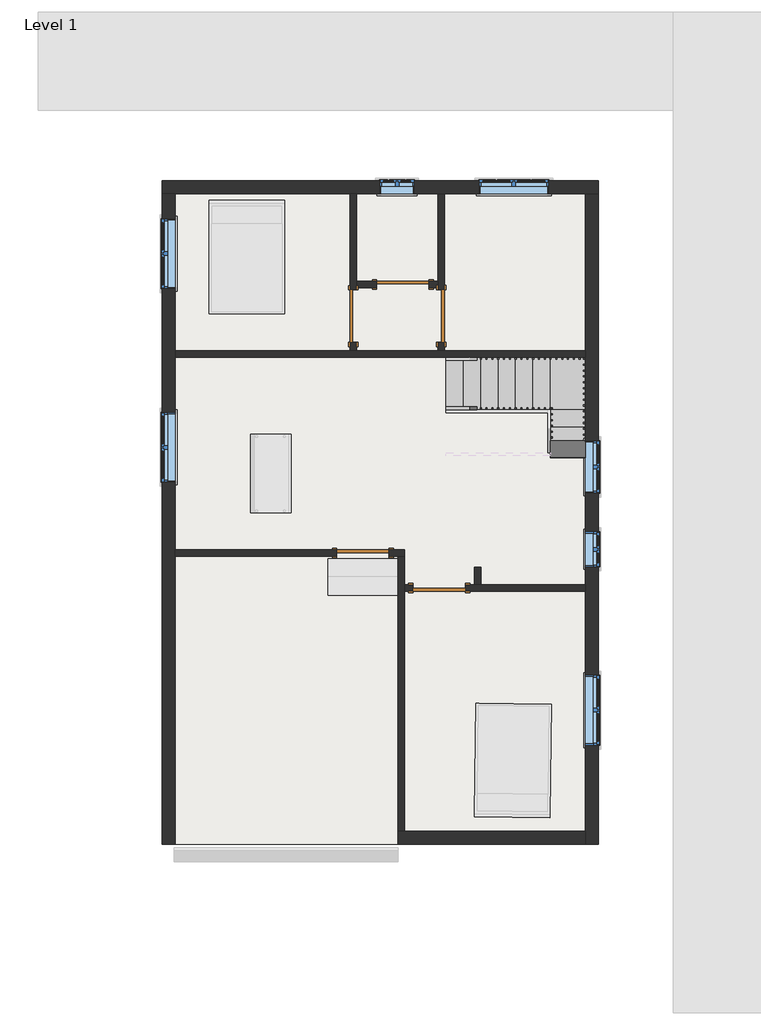
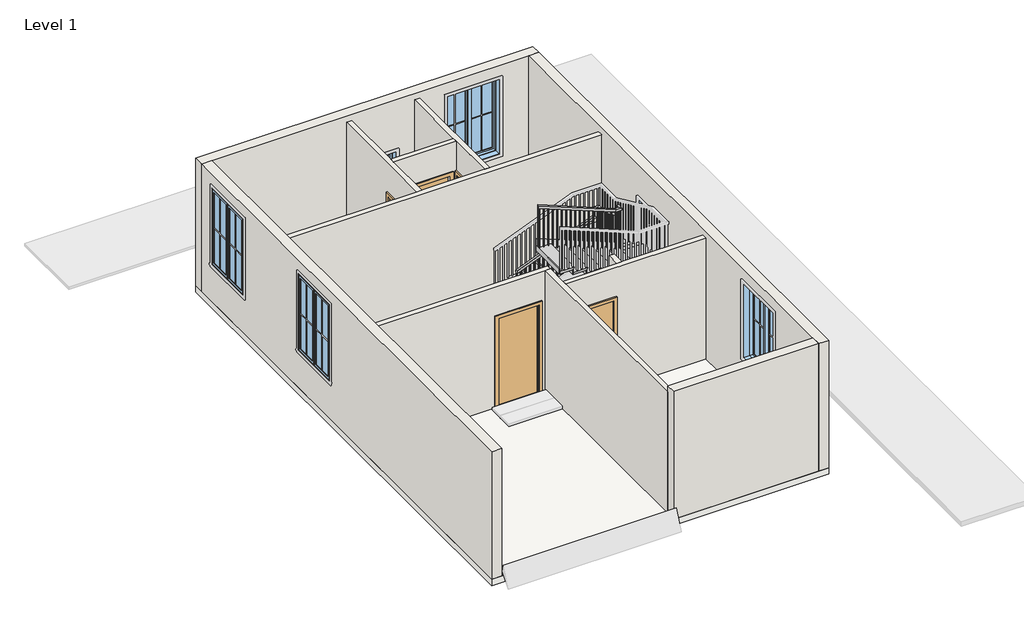
# One storey, part 1 of 2: 12 walls, 7 windows, 5 doors, 1 railing, 1 slab, 1 stair flight.
"""IFC4 building model written with IfcOpenShell, lengths in millimetres."""

from ifc_helpers import new_model, si_unit, frame, origin, origin_with_axes, place, context, project, spatial, polyline, outline, extrude, faceted_brep, transform, mapped, element, save
from components import door_e5f9f3c4, door_305aa2a5, stair_flight_8b794a03, window_c417fced, window_79f73a1a, window_6ca1769e

model = new_model("IFC4")

# Units and contexts
model_context = context("Model", 3, world=origin())
ifc_project = project(units=[si_unit("LENGTHUNIT", "METRE", prefix="MILLI")], contexts=[model_context])

# Site, building, storey
site = spatial("IfcSite", under=ifc_project)
building = spatial("IfcBuilding", under=site)
storey = spatial("IfcBuildingStorey", under=building, Name="Level 1", Elevation=0.0)

# Doors
placement = place(None, origin())
door_shape = door_e5f9f3c4(model_context)
element("IfcDoor", 1, ObjectType="Single-Flush : 36\" x 84\"", at=placement, inside=storey, context=model_context, shape_type="MappedRepresentation", body=[
    mapped(door_shape, transform((5727.7, 12245.5823212, 0.0), x_axis=(1.0, 0.0, 0.0), y_axis=(0.0, 1.0, 0.0), z_axis=(0.0, 0.0, 1.0))),
])
element("IfcDoor", 2, ObjectType="Single-Flush : 36\" x 84\"", at=placement, inside=storey, context=model_context, shape_type="MappedRepresentation", body=[
    mapped(door_shape, transform((6394.45, 11693.1323212, 0.0), x_axis=(0.0, -1.0, 0.0), y_axis=(1.0, 0.0, 0.0), z_axis=(0.0, 0.0, 1.0))),
])
element("IfcDoor", 3, ObjectType="Single-Flush : 36\" x 84\"", at=placement, inside=storey, context=model_context, shape_type="MappedRepresentation", body=[
    mapped(door_shape, transform((6362.7, 6949.6823212, 0.0), x_axis=(-1.0, 0.0, 0.0), y_axis=(0.0, -1.0, 0.0), z_axis=(0.0, 0.0, 1.0))),
])
element("IfcDoor", 4, ObjectType="Single-Flush : 36\" x 84\"", at=placement, inside=storey, context=model_context, shape_type="MappedRepresentation", body=[
    mapped(door_shape, transform((5029.2, 7559.2823212, 0.0), x_axis=(1.0, 0.0, 0.0), y_axis=(0.0, 1.0, 0.0), z_axis=(0.0, 0.0, 1.0))),
])
door_2_shape = door_305aa2a5(model_context)
element("IfcDoor", 5, ObjectType="Single-Flush : 36\" x 84\"", at=placement, inside=storey, context=model_context, shape_type="MappedRepresentation", body=[
    mapped(door_2_shape, transform((4857.75, 11689.9573212, 0.0), x_axis=(0.0, -1.0, 0.0), y_axis=(1.0, 0.0, 0.0), z_axis=(0.0, 0.0, 1.0))),
])

# Railing
element("IfcRailing", 6, ObjectType="Handrail - Rectangular", at=placement, inside=storey, context=model_context, shape_type="SolidModel", body=[
    faceted_brep([(6477.0, 10105.6323212, 1036.32), (6477.0, 10105.6323212, 981.6067256), (6477.0, 10054.8323212, 981.6067256), (6477.0, 10054.8323212, 1036.32), (8229.6, 10105.6323212, 1737.36), (8280.4, 10105.6323212, 1702.9667256), (8280.4, 10054.8323212, 1702.9667256), (8229.6, 10054.8323212, 1737.36), (8229.6, 10105.6323212, 1924.5942857), (8280.4, 10105.6323212, 1873.7942857), (8280.4, 10054.8323212, 1873.7942857), (8229.6, 10054.8323212, 1924.5942857), (8356.6, 10105.6323212, 1924.5942857), (8356.6, 10105.6323212, 1873.7942857), (8305.8, 10054.8323212, 1873.7942857), (8305.8, 10054.8323212, 1924.5942857), (8356.6, 9978.6323212, 1924.5942857), (8356.6, 9967.5713743, 1873.7942857), (8305.8, 9967.5713743, 1873.7942857), (8305.8, 9978.6323212, 1924.5942857), (8356.6, 9330.9323212, 2220.6857143), (8356.6, 9280.1323212, 2188.0521386), (8305.8, 9280.1323212, 2188.0521386), (8305.8, 9330.9323212, 2220.6857143), (8356.6, 9330.9323212, 2407.92), (8356.6, 9280.1323212, 2357.12), (8305.8, 9280.1323212, 2357.12), (8305.8, 9330.9323212, 2407.92), (8356.6, 9203.9323212, 2407.92), (8356.6, 9203.9323212, 2357.12), (8305.8, 9254.7323212, 2357.12), (8305.8, 9254.7323212, 2407.92), (8229.6, 9203.9323212, 2407.92), (8219.8168139, 9203.9323212, 2357.12), (8219.8168139, 9254.7323212, 2357.12), (8229.6, 9254.7323212, 2407.92), (6477.0, 9203.9323212, 3108.96), (6477.0, 9254.7323212, 3108.96), (6477.0, 9254.7323212, 3054.2467256), (6477.0, 9203.9323212, 3054.2467256)], [[[0, 1, 2, 3]], [[1, 0, 4, 5]], [[2, 1, 5, 6]], [[3, 2, 6, 7]], [[0, 3, 7, 4]], [[5, 4, 8, 9]], [[6, 5, 9, 10]], [[7, 6, 10, 11]], [[4, 7, 11, 8]], [[9, 8, 12, 13]], [[10, 9, 13, 14]], [[11, 10, 14, 15]], [[8, 11, 15, 12]], [[13, 12, 16, 17]], [[14, 13, 17, 18]], [[15, 14, 18, 19]], [[12, 15, 19, 16]], [[17, 16, 20, 21]], [[18, 17, 21, 22]], [[19, 18, 22, 23]], [[16, 19, 23, 20]], [[21, 20, 24, 25]], [[22, 21, 25, 26]], [[23, 22, 26, 27]], [[20, 23, 27, 24]], [[25, 24, 28, 29]], [[26, 25, 29, 30]], [[27, 26, 30, 31]], [[24, 27, 31, 28]], [[29, 28, 32, 33]], [[30, 29, 33, 34]], [[31, 30, 34, 35]], [[28, 31, 35, 32]], [[36, 37, 38, 39]], [[33, 32, 36, 39]], [[34, 33, 39, 38]], [[35, 34, 38, 37]], [[32, 35, 37, 36]]]),
    extrude(outline(polyline([(3040.2767256, 6511.925), (3047.8967256, 6492.875), (2072.64, 6492.875), (2072.64, 6511.925), (3040.2767256, 6511.925)])), frame((0.0, 9219.8073212, 0.0), z_axis=(0.0, 1.0, 0.0), x_axis=(0.0, 0.0, 1.0)), (0.0, 0.0, 1.0), 19.05),
    extrude(outline(polyline([(2999.6367256, 6613.525), (3007.2567256, 6594.475), (2072.64, 6594.475), (2072.64, 6613.525), (2999.6367256, 6613.525)])), frame((0.0, 9219.8073212, 0.0), z_axis=(0.0, 1.0, 0.0), x_axis=(0.0, 0.0, 1.0)), (0.0, 0.0, 1.0), 19.05),
    extrude(outline(polyline([(2958.9967256, 6715.125), (2966.6167256, 6696.075), (2072.64, 6696.075), (2072.64, 6715.125), (2958.9967256, 6715.125)])), frame((0.0, 9219.8073212, 0.0), z_axis=(0.0, 1.0, 0.0), x_axis=(0.0, 0.0, 1.0)), (0.0, 0.0, 1.0), 19.05),
    extrude(outline(polyline([(2918.3567256, 6816.725), (2925.9767256, 6797.675), (1950.72, 6797.675), (1950.72, 6816.725), (2918.3567256, 6816.725)])), frame((0.0, 9219.8073212, 0.0), z_axis=(0.0, 1.0, 0.0), x_axis=(0.0, 0.0, 1.0)), (0.0, 0.0, 1.0), 19.05),
    extrude(outline(polyline([(2877.7167256, 6918.325), (2885.3367256, 6899.275), (1950.72, 6899.275), (1950.72, 6918.325), (2877.7167256, 6918.325)])), frame((0.0, 9219.8073212, 0.0), z_axis=(0.0, 1.0, 0.0), x_axis=(0.0, 0.0, 1.0)), (0.0, 0.0, 1.0), 19.05),
    extrude(outline(polyline([(2837.0767256, 7019.925), (2844.6967256, 7000.875), (1950.72, 7000.875), (1950.72, 7019.925), (2837.0767256, 7019.925)])), frame((0.0, 9219.8073212, 0.0), z_axis=(0.0, 1.0, 0.0), x_axis=(0.0, 0.0, 1.0)), (0.0, 0.0, 1.0), 19.05),
    extrude(outline(polyline([(2796.4367256, 7121.525), (2804.0567256, 7102.475), (1828.8, 7102.475), (1828.8, 7121.525), (2796.4367256, 7121.525)])), frame((0.0, 9219.8073212, 0.0), z_axis=(0.0, 1.0, 0.0), x_axis=(0.0, 0.0, 1.0)), (0.0, 0.0, 1.0), 19.05),
    extrude(outline(polyline([(2755.7967256, 7223.125), (2763.4167256, 7204.075), (1828.8, 7204.075), (1828.8, 7223.125), (2755.7967256, 7223.125)])), frame((0.0, 9219.8073212, 0.0), z_axis=(0.0, 1.0, 0.0), x_axis=(0.0, 0.0, 1.0)), (0.0, 0.0, 1.0), 19.05),
    extrude(outline(polyline([(2715.1567256, 7324.725), (2722.7767256, 7305.675), (1828.8, 7305.675), (1828.8, 7324.725), (2715.1567256, 7324.725)])), frame((0.0, 9219.8073212, 0.0), z_axis=(0.0, 1.0, 0.0), x_axis=(0.0, 0.0, 1.0)), (0.0, 0.0, 1.0), 19.05),
    extrude(outline(polyline([(2674.5167256, 7426.325), (2682.1367256, 7407.275), (1706.88, 7407.275), (1706.88, 7426.325), (2674.5167256, 7426.325)])), frame((0.0, 9219.8073212, 0.0), z_axis=(0.0, 1.0, 0.0), x_axis=(0.0, 0.0, 1.0)), (0.0, 0.0, 1.0), 19.05),
    extrude(outline(polyline([(2633.8767256, 7527.925), (2641.4967256, 7508.875), (1706.88, 7508.875), (1706.88, 7527.925), (2633.8767256, 7527.925)])), frame((0.0, 9219.8073212, 0.0), z_axis=(0.0, 1.0, 0.0), x_axis=(0.0, 0.0, 1.0)), (0.0, 0.0, 1.0), 19.05),
    extrude(outline(polyline([(2593.2367256, 7629.525), (2600.8567256, 7610.475), (1706.88, 7610.475), (1706.88, 7629.525), (2593.2367256, 7629.525)])), frame((0.0, 9219.8073212, 0.0), z_axis=(0.0, 1.0, 0.0), x_axis=(0.0, 0.0, 1.0)), (0.0, 0.0, 1.0), 19.05),
    extrude(outline(polyline([(2552.5967256, 7731.125), (2560.2167256, 7712.075), (1584.96, 7712.075), (1584.96, 7731.125), (2552.5967256, 7731.125)])), frame((0.0, 9219.8073212, 0.0), z_axis=(0.0, 1.0, 0.0), x_axis=(0.0, 0.0, 1.0)), (0.0, 0.0, 1.0), 19.05),
    extrude(outline(polyline([(2511.9567256, 7832.725), (2519.5767256, 7813.675), (1584.96, 7813.675), (1584.96, 7832.725), (2511.9567256, 7832.725)])), frame((0.0, 9219.8073212, 0.0), z_axis=(0.0, 1.0, 0.0), x_axis=(0.0, 0.0, 1.0)), (0.0, 0.0, 1.0), 19.05),
    extrude(outline(polyline([(2471.3167256, 7934.325), (2478.9367256, 7915.275), (1584.96, 7915.275), (1584.96, 7934.325), (2471.3167256, 7934.325)])), frame((0.0, 9219.8073212, 0.0), z_axis=(0.0, 1.0, 0.0), x_axis=(0.0, 0.0, 1.0)), (0.0, 0.0, 1.0), 19.05),
    extrude(outline(polyline([(2430.6767256, 8035.925), (2438.2967256, 8016.875), (1463.04, 8016.875), (1463.04, 8035.925), (2430.6767256, 8035.925)])), frame((0.0, 9219.8073212, 0.0), z_axis=(0.0, 1.0, 0.0), x_axis=(0.0, 0.0, 1.0)), (0.0, 0.0, 1.0), 19.05),
    extrude(outline(polyline([(2390.0367256, 8137.525), (2397.6567256, 8118.475), (1463.04, 8118.475), (1463.04, 8137.525), (2390.0367256, 8137.525)])), frame((0.0, 9219.8073212, 0.0), z_axis=(0.0, 1.0, 0.0), x_axis=(0.0, 0.0, 1.0)), (0.0, 0.0, 1.0), 19.05),
    extrude(outline(polyline([(2349.3967256, 8239.125), (2357.0167256, 8220.075), (1463.04, 8220.075), (1463.04, 8239.125), (2349.3967256, 8239.125)])), frame((0.0, 9219.8073212, 0.0), z_axis=(0.0, 1.0, 0.0), x_axis=(0.0, 0.0, 1.0)), (0.0, 0.0, 1.0), 19.05),
    extrude(outline(polyline([(8321.675, 9276.9573212), (8340.725, 9276.9573212), (8340.725, 9257.9073212), (8321.675, 9257.9073212), (8321.675, 9276.9573212)])), frame((0.0, 0.0, 1219.2), z_axis=(0.0, 0.0, 1.0), x_axis=(1.0, 0.0, 0.0)), (0.0, 0.0, 1.0), 1137.92),
    extrude(outline(polyline([(9359.5073212, 2151.7664243), (9378.5573212, 2143.0578528), (9378.5573212, 1219.2), (9359.5073212, 1219.2), (9359.5073212, 2151.7664243)])), frame((8321.675, 0.0, 0.0), z_axis=(1.0, 0.0, 0.0), x_axis=(0.0, 1.0, 0.0)), (0.0, 0.0, 1.0), 19.05),
    extrude(outline(polyline([(9461.1073212, 2105.32071), (9480.1573212, 2096.6121386), (9480.1573212, 1219.2), (9461.1073212, 1219.2), (9461.1073212, 2105.32071)])), frame((8321.675, 0.0, 0.0), z_axis=(1.0, 0.0, 0.0), x_axis=(0.0, 1.0, 0.0)), (0.0, 0.0, 1.0), 19.05),
    extrude(outline(polyline([(9562.7073212, 2058.8749957), (9581.7573212, 2050.1664243), (9581.7573212, 1097.28), (9562.7073212, 1097.28), (9562.7073212, 2058.8749957)])), frame((8321.675, 0.0, 0.0), z_axis=(1.0, 0.0, 0.0), x_axis=(0.0, 1.0, 0.0)), (0.0, 0.0, 1.0), 19.05),
    extrude(outline(polyline([(9664.3073212, 2012.4292814), (9683.3573212, 2003.72071), (9683.3573212, 1097.28), (9664.3073212, 1097.28), (9664.3073212, 2012.4292814)])), frame((8321.675, 0.0, 0.0), z_axis=(1.0, 0.0, 0.0), x_axis=(0.0, 1.0, 0.0)), (0.0, 0.0, 1.0), 19.05),
    extrude(outline(polyline([(9765.9073212, 1965.9835671), (9784.9573212, 1957.2749957), (9784.9573212, 975.36), (9765.9073212, 975.36), (9765.9073212, 1965.9835671)])), frame((8321.675, 0.0, 0.0), z_axis=(1.0, 0.0, 0.0), x_axis=(0.0, 1.0, 0.0)), (0.0, 0.0, 1.0), 19.05),
    extrude(outline(polyline([(9867.5073212, 1919.5378528), (9886.5573212, 1910.8292814), (9886.5573212, 975.36), (9867.5073212, 975.36), (9867.5073212, 1919.5378528)])), frame((8321.675, 0.0, 0.0), z_axis=(1.0, 0.0, 0.0), x_axis=(0.0, 1.0, 0.0)), (0.0, 0.0, 1.0), 19.05),
    extrude(outline(polyline([(9969.1073212, 1873.0921386), (9988.1573212, 1864.3835671), (9988.1573212, 975.36), (9969.1073212, 975.36), (9969.1073212, 1873.0921386)])), frame((8321.675, 0.0, 0.0), z_axis=(1.0, 0.0, 0.0), x_axis=(0.0, 1.0, 0.0)), (0.0, 0.0, 1.0), 19.05),
    extrude(outline(polyline([(8296.275, 10070.7073212), (8296.275, 10089.7573212), (8315.325, 10089.7573212), (8315.325, 10070.7073212), (8296.275, 10070.7073212)])), frame((0.0, 0.0, 853.44), z_axis=(0.0, 0.0, 1.0), x_axis=(1.0, 0.0, 0.0)), (0.0, 0.0, 1.0), 1020.3542857),
    extrude(outline(polyline([(1676.2967256, 8213.725), (1668.6767256, 8194.675), (731.52, 8194.675), (731.52, 8213.725), (1676.2967256, 8213.725)])), frame((0.0, 10070.7073212, 0.0), z_axis=(0.0, 1.0, 0.0), x_axis=(0.0, 0.0, 1.0)), (0.0, 0.0, 1.0), 19.05),
    extrude(outline(polyline([(1635.6567256, 8112.125), (1628.0367256, 8093.075), (731.52, 8093.075), (731.52, 8112.125), (1635.6567256, 8112.125)])), frame((0.0, 10070.7073212, 0.0), z_axis=(0.0, 1.0, 0.0), x_axis=(0.0, 0.0, 1.0)), (0.0, 0.0, 1.0), 19.05),
    extrude(outline(polyline([(1595.0167256, 8010.525), (1587.3967256, 7991.475), (731.52, 7991.475), (731.52, 8010.525), (1595.0167256, 8010.525)])), frame((0.0, 10070.7073212, 0.0), z_axis=(0.0, 1.0, 0.0), x_axis=(0.0, 0.0, 1.0)), (0.0, 0.0, 1.0), 19.05),
    extrude(outline(polyline([(1554.3767256, 7908.925), (1546.7567256, 7889.875), (609.6, 7889.875), (609.6, 7908.925), (1554.3767256, 7908.925)])), frame((0.0, 10070.7073212, 0.0), z_axis=(0.0, 1.0, 0.0), x_axis=(0.0, 0.0, 1.0)), (0.0, 0.0, 1.0), 19.05),
    extrude(outline(polyline([(1513.7367256, 7807.325), (1506.1167256, 7788.275), (609.6, 7788.275), (609.6, 7807.325), (1513.7367256, 7807.325)])), frame((0.0, 10070.7073212, 0.0), z_axis=(0.0, 1.0, 0.0), x_axis=(0.0, 0.0, 1.0)), (0.0, 0.0, 1.0), 19.05),
    extrude(outline(polyline([(1473.0967256, 7705.725), (1465.4767256, 7686.675), (609.6, 7686.675), (609.6, 7705.725), (1473.0967256, 7705.725)])), frame((0.0, 10070.7073212, 0.0), z_axis=(0.0, 1.0, 0.0), x_axis=(0.0, 0.0, 1.0)), (0.0, 0.0, 1.0), 19.05),
    extrude(outline(polyline([(1432.4567256, 7604.125), (1424.8367256, 7585.075), (487.68, 7585.075), (487.68, 7604.125), (1432.4567256, 7604.125)])), frame((0.0, 10070.7073212, 0.0), z_axis=(0.0, 1.0, 0.0), x_axis=(0.0, 0.0, 1.0)), (0.0, 0.0, 1.0), 19.05),
    extrude(outline(polyline([(1391.8167256, 7502.525), (1384.1967256, 7483.475), (487.68, 7483.475), (487.68, 7502.525), (1391.8167256, 7502.525)])), frame((0.0, 10070.7073212, 0.0), z_axis=(0.0, 1.0, 0.0), x_axis=(0.0, 0.0, 1.0)), (0.0, 0.0, 1.0), 19.05),
    extrude(outline(polyline([(1351.1767256, 7400.925), (1343.5567256, 7381.875), (487.68, 7381.875), (487.68, 7400.925), (1351.1767256, 7400.925)])), frame((0.0, 10070.7073212, 0.0), z_axis=(0.0, 1.0, 0.0), x_axis=(0.0, 0.0, 1.0)), (0.0, 0.0, 1.0), 19.05),
    extrude(outline(polyline([(1310.5367256, 7299.325), (1302.9167256, 7280.275), (365.76, 7280.275), (365.76, 7299.325), (1310.5367256, 7299.325)])), frame((0.0, 10070.7073212, 0.0), z_axis=(0.0, 1.0, 0.0), x_axis=(0.0, 0.0, 1.0)), (0.0, 0.0, 1.0), 19.05),
    extrude(outline(polyline([(1269.8967256, 7197.725), (1262.2767256, 7178.675), (365.76, 7178.675), (365.76, 7197.725), (1269.8967256, 7197.725)])), frame((0.0, 10070.7073212, 0.0), z_axis=(0.0, 1.0, 0.0), x_axis=(0.0, 0.0, 1.0)), (0.0, 0.0, 1.0), 19.05),
    extrude(outline(polyline([(1229.2567256, 7096.125), (1221.6367256, 7077.075), (365.76, 7077.075), (365.76, 7096.125), (1229.2567256, 7096.125)])), frame((0.0, 10070.7073212, 0.0), z_axis=(0.0, 1.0, 0.0), x_axis=(0.0, 0.0, 1.0)), (0.0, 0.0, 1.0), 19.05),
    extrude(outline(polyline([(1188.6167256, 6994.525), (1180.9967256, 6975.475), (243.84, 6975.475), (243.84, 6994.525), (1188.6167256, 6994.525)])), frame((0.0, 10070.7073212, 0.0), z_axis=(0.0, 1.0, 0.0), x_axis=(0.0, 0.0, 1.0)), (0.0, 0.0, 1.0), 19.05),
    extrude(outline(polyline([(1147.9767256, 6892.925), (1140.3567256, 6873.875), (243.84, 6873.875), (243.84, 6892.925), (1147.9767256, 6892.925)])), frame((0.0, 10070.7073212, 0.0), z_axis=(0.0, 1.0, 0.0), x_axis=(0.0, 0.0, 1.0)), (0.0, 0.0, 1.0), 19.05),
    extrude(outline(polyline([(1107.3367256, 6791.325), (1099.7167256, 6772.275), (243.84, 6772.275), (243.84, 6791.325), (1107.3367256, 6791.325)])), frame((0.0, 10070.7073212, 0.0), z_axis=(0.0, 1.0, 0.0), x_axis=(0.0, 0.0, 1.0)), (0.0, 0.0, 1.0), 19.05),
    extrude(outline(polyline([(1066.6967256, 6689.725), (1059.0767256, 6670.675), (121.92, 6670.675), (121.92, 6689.725), (1066.6967256, 6689.725)])), frame((0.0, 10070.7073212, 0.0), z_axis=(0.0, 1.0, 0.0), x_axis=(0.0, 0.0, 1.0)), (0.0, 0.0, 1.0), 19.05),
    extrude(outline(polyline([(1026.0567256, 6588.125), (1018.4367256, 6569.075), (121.92, 6569.075), (121.92, 6588.125), (1026.0567256, 6588.125)])), frame((0.0, 10070.7073212, 0.0), z_axis=(0.0, 1.0, 0.0), x_axis=(0.0, 0.0, 1.0)), (0.0, 0.0, 1.0), 19.05),
    extrude(outline(polyline([(8321.675, 9238.8573212), (8340.725, 9238.8573212), (8340.725, 9219.8073212), (8321.675, 9219.8073212), (8321.675, 9238.8573212)])), frame((0.0, 0.0, 1341.12), z_axis=(0.0, 0.0, 1.0), x_axis=(1.0, 0.0, 0.0)), (0.0, 0.0, 1.0), 1016.0),
    extrude(outline(polyline([(8321.675, 10070.7073212), (8321.675, 10089.7573212), (8340.725, 10089.7573212), (8340.725, 10070.7073212), (8321.675, 10070.7073212)])), frame((0.0, 0.0, 853.44), z_axis=(0.0, 0.0, 1.0), x_axis=(1.0, 0.0, 0.0)), (0.0, 0.0, 1.0), 1020.3542857),
    extrude(outline(polyline([(3046.6267256, 6496.05), (3054.2467256, 6477.0), (2072.64, 6477.0), (2072.64, 6496.05), (3046.6267256, 6496.05)])), frame((0.0, 9219.8073212, 0.0), z_axis=(0.0, 1.0, 0.0), x_axis=(0.0, 0.0, 1.0)), (0.0, 0.0, 1.0), 19.05),
    extrude(outline(polyline([(989.2267256, 6496.05), (981.6067256, 6477.0), (121.92, 6477.0), (121.92, 6496.05), (989.2267256, 6496.05)])), frame((0.0, 10070.7073212, 0.0), z_axis=(0.0, 1.0, 0.0), x_axis=(0.0, 0.0, 1.0)), (0.0, 0.0, 1.0), 19.05),
])

# Slab
element("IfcSlab", 7, ObjectType="Generic - 12\"", at=placement, inside=storey, context=model_context, shape_type="SweptSolid", body=[
    extrude(outline(polyline([(9144.0, 14055.3323212), (9144.0, 2472.9323212), (1524.0, 2472.9323212), (1524.0, 14055.3323212), (9144.0, 14055.3323212)])), frame((0.0, 0.0, -152.4), z_axis=(0.0, 0.0, 1.0), x_axis=(1.0, 0.0, 0.0)), (0.0, 0.0, 1.0), 152.4),
])

# Stair flight
stair_flight_shape = stair_flight_8b794a03(model_context)
element("IfcStairFlight", 8, ObjectType="2\" Tread 1\" Nosing 1/4\" Riser", at=placement, inside=storey, context=model_context, shape_type="MappedRepresentation", body=[
    mapped(stair_flight_shape, transform((0.0, 0.0, 0.0), x_axis=(1.0, 0.0, 0.0), y_axis=(0.0, 1.0, 0.0), z_axis=(0.0, 0.0, 1.0))),
])

# Walls
element("IfcWall", 9, ObjectType="Generic - 5\"", at=placement, inside=storey, context=model_context, shape_type="Brep", body=[
    faceted_brep([(4800.6, 11232.7573212, 2133.6), (4800.6, 11232.7573212, 0.0), (4800.6, 11083.5323212, 0.0), (4800.6, 11083.5323212, 2895.6), (4800.6, 13826.7323212, 2895.6), (4800.6, 13826.7323212, 0.0), (4800.6, 12147.1573212, 0.0), (4800.6, 12147.1573212, 2133.6), (4914.9, 11083.5323212, 0.0), (4914.9, 11232.7573212, 0.0), (4914.9, 11232.7573212, 2133.6), (4914.9, 12147.1573212, 2133.6), (4914.9, 12147.1573212, 0.0), (4914.9, 12188.4323212, 0.0), (4914.9, 12302.7323212, 0.0), (4914.9, 13826.7323212, 0.0), (4914.9, 13826.7323212, 2895.6), (4914.9, 12302.7323212, 2895.6), (4914.9, 12188.4323212, 2895.6), (4914.9, 11083.5323212, 2895.6)], [[[0, 1, 2, 3, 4, 5, 6, 7]], [[8, 9, 10, 11, 12, 13, 14, 15, 16, 17, 18, 19]], [[6, 5, 15, 14, 13, 12]], [[2, 1, 9, 8]], [[5, 4, 16, 15]], [[3, 2, 8, 19]], [[10, 9, 1, 0]], [[11, 10, 0, 7]], [[12, 11, 7, 6]], [[4, 3, 19, 18, 17, 16]]]),
])
element("IfcWall", 10, ObjectType="Generic - 5\"", at=placement, inside=storey, context=model_context, shape_type="Brep", body=[
    faceted_brep([(6337.3, 11235.9323212, 2133.6), (6337.3, 11235.9323212, 0.0), (6337.3, 11083.5323212, 0.0), (6337.3, 11083.5323212, 2895.6), (6337.3, 12188.4323212, 2895.6), (6337.3, 12302.7323212, 2895.6), (6337.3, 13826.7323212, 2895.6), (6337.3, 13826.7323212, 0.0), (6337.3, 12302.7323212, 0.0), (6337.3, 12188.4323212, 0.0), (6337.3, 12150.3323212, 0.0), (6337.3, 12150.3323212, 2133.6), (6451.6, 11083.5323212, 0.0), (6451.6, 11235.9323212, 0.0), (6451.6, 11235.9323212, 2133.6), (6451.6, 12150.3323212, 2133.6), (6451.6, 12150.3323212, 0.0), (6451.6, 13826.7323212, 0.0), (6451.6, 13826.7323212, 2895.6), (6451.6, 11083.5323212, 2895.6)], [[[0, 1, 2, 3, 4, 5, 6, 7, 8, 9, 10, 11]], [[12, 13, 14, 15, 16, 17, 18, 19]], [[2, 1, 13, 12]], [[10, 9, 8, 7, 17, 16]], [[7, 6, 18, 17]], [[3, 2, 12, 19]], [[14, 13, 1, 0]], [[15, 14, 0, 11]], [[16, 15, 11, 10]], [[6, 5, 4, 3, 19, 18]]]),
])
element("IfcWall", 11, ObjectType="Generic - 5\"", at=placement, inside=storey, context=model_context, shape_type="SweptSolid", body=[
    extrude(outline(polyline([(2133.6, 6184.9), (0.0, 6184.9), (0.0, 6337.3), (2895.6, 6337.3), (2895.6, 4914.9), (0.0, 4914.9), (0.0, 5270.5), (2133.6, 5270.5), (2133.6, 6184.9)])), frame((0.0, 12188.4323212, 0.0), z_axis=(0.0, 1.0, 0.0), x_axis=(0.0, 0.0, 1.0)), (0.0, 0.0, 1.0), 114.3),
])
element("IfcWall", 12, ObjectType="Generic - 5\"", at=placement, inside=storey, context=model_context, shape_type="Brep", body=[
    faceted_brep([(1752.6, 10969.2323212, 0.0), (8915.4, 10969.2323212, 0.0), (8915.4, 10969.2323212, 2895.6), (1752.6, 10969.2323212, 2895.6), (1752.6, 11083.5323212, 0.0), (1752.6, 11083.5323212, 2895.6), (4800.6, 11083.5323212, 2895.6), (4914.9, 11083.5323212, 2895.6), (6337.3, 11083.5323212, 2895.6), (6451.6, 11083.5323212, 2895.6), (8915.4, 11083.5323212, 2895.6), (8915.4, 11083.5323212, 0.0), (6451.6, 11083.5323212, 0.0), (6337.3, 11083.5323212, 0.0), (4914.9, 11083.5323212, 0.0), (4800.6, 11083.5323212, 0.0)], [[[0, 1, 2, 3]], [[4, 5, 6, 7, 8, 9, 10, 11, 12, 13, 14, 15]], [[1, 0, 4, 15, 14, 13, 12, 11]], [[2, 1, 11, 10]], [[0, 3, 5, 4]], [[3, 2, 10, 9, 8, 7, 6, 5]]]),
])
element("IfcWall", 13, ObjectType="Generic - 5\"", at=placement, inside=storey, context=model_context, shape_type="Brep", body=[
    faceted_brep([(5486.4, 7502.1323212, 2133.6), (5486.4, 7502.1323212, 0.0), (5638.8, 7502.1323212, 0.0), (5753.1, 7502.1323212, 0.0), (5753.1, 7502.1323212, 2895.6), (5638.8, 7502.1323212, 2895.6), (1752.6, 7502.1323212, 2895.6), (1752.6, 7502.1323212, 0.0), (4572.0, 7502.1323212, 0.0), (4572.0, 7502.1323212, 2133.6), (5753.1, 7616.4323212, 0.0), (5486.4, 7616.4323212, 0.0), (5486.4, 7616.4323212, 2133.6), (4572.0, 7616.4323212, 2133.6), (4572.0, 7616.4323212, 0.0), (1752.6, 7616.4323212, 0.0), (1752.6, 7616.4323212, 2895.6), (5753.1, 7616.4323212, 2895.6)], [[[0, 1, 2, 3, 4, 5, 6, 7, 8, 9]], [[10, 11, 12, 13, 14, 15, 16, 17]], [[8, 7, 15, 14]], [[3, 2, 1, 11, 10]], [[7, 6, 16, 15]], [[4, 3, 10, 17]], [[12, 11, 1, 0]], [[13, 12, 0, 9]], [[14, 13, 9, 8]], [[6, 5, 4, 17, 16]]]),
])
element("IfcWall", 14, ObjectType="Generic - 5\"", at=placement, inside=storey, context=model_context, shape_type="Brep", body=[
    faceted_brep([(5638.8, 7502.1323212, 0.0), (5638.8, 2700.7084466, 0.0), (5638.8, 2700.7084466, 2895.6), (5638.8, 7502.1323212, 2895.6), (5753.1, 7502.1323212, 0.0), (5753.1, 7502.1323212, 2895.6), (5753.1, 7006.8323212, 2895.6), (5753.1, 6892.5323212, 2895.6), (5753.1, 2700.7084466, 2895.6), (5753.1, 2700.7084466, 0.0), (5753.1, 6892.5323212, 0.0), (5753.1, 7006.8323212, 0.0)], [[[0, 1, 2, 3]], [[4, 5, 6, 7, 8, 9, 10, 11]], [[1, 0, 4, 11, 10, 9]], [[0, 3, 5, 4]], [[2, 1, 9, 8]], [[3, 2, 8, 7, 6, 5]]]),
])
element("IfcWall", 15, ObjectType="Generic - 5\"", at=placement, inside=storey, context=model_context, shape_type="Brep", body=[
    faceted_brep([(5905.5, 7006.8323212, 2133.6), (5905.5, 7006.8323212, 0.0), (5753.1, 7006.8323212, 0.0), (5753.1, 7006.8323212, 2895.6), (6972.3, 7006.8323212, 2895.6), (7086.6, 7006.8323212, 2895.6), (8915.4, 7006.8323212, 2895.6), (8915.4, 7006.8323212, 0.0), (7086.6, 7006.8323212, 0.0), (6972.3, 7006.8323212, 0.0), (6819.9, 7006.8323212, 0.0), (6819.9, 7006.8323212, 2133.6), (5753.1, 6892.5323212, 0.0), (5905.5, 6892.5323212, 0.0), (5905.5, 6892.5323212, 2133.6), (6819.9, 6892.5323212, 2133.6), (6819.9, 6892.5323212, 0.0), (8915.4, 6892.5323212, 0.0), (8915.4, 6892.5323212, 2895.6), (5753.1, 6892.5323212, 2895.6)], [[[0, 1, 2, 3, 4, 5, 6, 7, 8, 9, 10, 11]], [[12, 13, 14, 15, 16, 17, 18, 19]], [[2, 1, 13, 12]], [[10, 9, 8, 7, 17, 16]], [[7, 6, 18, 17]], [[3, 2, 12, 19]], [[14, 13, 1, 0]], [[15, 14, 0, 11]], [[16, 15, 11, 10]], [[6, 5, 4, 3, 19, 18]]]),
])
element("IfcWall", 16, ObjectType="Generic - 5\"", at=placement, inside=storey, context=model_context, shape_type="SweptSolid", body=[
    extrude(outline(polyline([(7086.6, 7311.6323212), (7086.6, 7006.8323212), (6972.3, 7006.8323212), (6972.3, 7311.6323212), (7086.6, 7311.6323212)])), origin_with_axes(), (0.0, 0.0, 1.0), 2895.6),
])
element("IfcWall", 17, ObjectType="Generic - 8\"", at=placement, inside=storey, context=model_context, shape_type="Brep", body=[
    faceted_brep([(1524.0, 13826.7323212, 0.0), (1752.6, 13826.7323212, 0.0), (4800.6, 13826.7323212, 0.0), (4914.9, 13826.7323212, 0.0), (6337.3, 13826.7323212, 0.0), (6451.6, 13826.7323212, 0.0), (8915.4, 13826.7323212, 0.0), (9144.0, 13826.7323212, 0.0), (9144.0, 13826.7323212, 3048.0), (8915.4, 13826.7323212, 3048.0), (1752.6, 13826.7323212, 3048.0), (1524.0, 13826.7323212, 3048.0), (8274.05, 13826.7323212, 2743.2), (8274.05, 13826.7323212, 914.4), (7054.85, 13826.7323212, 914.4), (7054.85, 13826.7323212, 2743.2), (5930.9, 13826.7323212, 1828.8), (5930.9, 13826.7323212, 914.4), (5321.3, 13826.7323212, 914.4), (5321.3, 13826.7323212, 1828.8), (1524.0, 14055.3323212, 0.0), (1524.0, 14055.3323212, 3048.0), (9144.0, 14055.3323212, 3048.0), (9144.0, 14055.3323212, 0.0), (8274.05, 14055.3323212, 2743.2), (7054.85, 14055.3323212, 2743.2), (7054.85, 14055.3323212, 914.4), (8274.05, 14055.3323212, 914.4), (5930.9, 14055.3323212, 1828.8), (5321.3, 14055.3323212, 1828.8), (5321.3, 14055.3323212, 914.4), (5930.9, 14055.3323212, 914.4)], [[[0, 1, 2, 3, 4, 5, 6, 7, 8, 9, 10, 11], [12, 13, 14, 15], [16, 17, 18, 19]], [[20, 21, 22, 23], [24, 25, 26, 27], [28, 29, 30, 31]], [[7, 6, 5, 4, 3, 2, 1, 0, 20, 23]], [[11, 10, 9, 8, 22, 21]], [[8, 7, 23, 22]], [[0, 11, 21, 20]], [[13, 12, 24, 27]], [[14, 13, 27, 26]], [[15, 14, 26, 25]], [[12, 15, 25, 24]], [[17, 16, 28, 31]], [[18, 17, 31, 30]], [[19, 18, 30, 29]], [[16, 19, 29, 28]]]),
])
element("IfcWall", 18, ObjectType="Generic - 8\"", at=placement, inside=storey, context=model_context, shape_type="Brep", body=[
    faceted_brep([(8915.4, 13826.7323212, 0.0), (8915.4, 11083.5323212, 0.0), (8915.4, 10969.2323212, 0.0), (8915.4, 7006.8323212, 0.0), (8915.4, 6892.5323212, 0.0), (8915.4, 2700.7084466, 0.0), (8915.4, 2472.1084466, 0.0), (8915.4, 2472.1084466, 3048.0), (8915.4, 2700.7084466, 3048.0), (8915.4, 13826.7323212, 3048.0), (8915.4, 4206.4823212, 2743.2), (8915.4, 4206.4823212, 914.4), (8915.4, 5425.6823212, 914.4), (8915.4, 5425.6823212, 2743.2), (8915.4, 7315.6010712, 1828.8), (8915.4, 7315.6010712, 914.4), (8915.4, 7925.2010712, 914.4), (8915.4, 7925.2010712, 1828.8), (8915.4, 8602.8899384, 2260.6), (8915.4, 8602.8899384, 914.4), (8915.4, 9517.2899384, 914.4), (8915.4, 9517.2899384, 2260.6), (9144.0, 13826.7323212, 0.0), (9144.0, 13826.7323212, 3048.0), (9144.0, 2472.1084466, 3048.0), (9144.0, 2472.1084466, 0.0), (9144.0, 4206.4823212, 2743.2), (9144.0, 5425.6823212, 2743.2), (9144.0, 5425.6823212, 914.4), (9144.0, 4206.4823212, 914.4), (9144.0, 7315.6010712, 1828.8), (9144.0, 7925.2010712, 1828.8), (9144.0, 7925.2010712, 914.4), (9144.0, 7315.6010712, 914.4), (9144.0, 8602.8899384, 2260.6), (9144.0, 9517.2899384, 2260.6), (9144.0, 9517.2899384, 914.4), (9144.0, 8602.8899384, 914.4)], [[[0, 1, 2, 3, 4, 5, 6, 7, 8, 9], [10, 11, 12, 13], [14, 15, 16, 17], [18, 19, 20, 21]], [[22, 23, 24, 25], [26, 27, 28, 29], [30, 31, 32, 33], [34, 35, 36, 37]], [[6, 5, 4, 3, 2, 1, 0, 22, 25]], [[9, 8, 7, 24, 23]], [[0, 9, 23, 22]], [[7, 6, 25, 24]], [[11, 10, 26, 29]], [[12, 11, 29, 28]], [[13, 12, 28, 27]], [[10, 13, 27, 26]], [[15, 14, 30, 33]], [[16, 15, 33, 32]], [[17, 16, 32, 31]], [[14, 17, 31, 30]], [[19, 18, 34, 37]], [[20, 19, 37, 36]], [[21, 20, 36, 35]], [[18, 21, 35, 34]]]),
])
element("IfcWall", 19, ObjectType="Generic - 8\"", at=placement, inside=storey, context=model_context, shape_type="Brep", body=[
    faceted_brep([(8915.4, 2700.7084466, 0.0), (5753.1, 2700.7084466, 0.0), (5638.8, 2700.7084466, 0.0), (5638.8, 2700.7084466, 2895.6), (5638.8, 2700.7084466, 3048.0), (8915.4, 2700.7084466, 3048.0), (8915.4, 2472.1084466, 0.0), (8915.4, 2472.1084466, 3048.0), (5638.8, 2472.1084466, 3048.0), (5638.8, 2472.1084466, 0.0)], [[[0, 1, 2, 3, 4, 5]], [[6, 7, 8, 9]], [[2, 1, 0, 6, 9]], [[4, 3, 2, 9, 8]], [[5, 4, 8, 7]], [[0, 5, 7, 6]]]),
])
element("IfcWall", 20, ObjectType="Generic - 8\"", at=placement, inside=storey, context=model_context, shape_type="Brep", body=[
    faceted_brep([(1752.6, 2472.9323212, 0.0), (1752.6, 7502.1323212, 0.0), (1752.6, 7616.4323212, 0.0), (1752.6, 10969.2323212, 0.0), (1752.6, 11083.5323212, 0.0), (1752.6, 13826.7323212, 0.0), (1752.6, 13826.7323212, 3048.0), (1752.6, 2472.9323212, 3048.0), (1752.6, 13390.2194306, 2743.2), (1752.6, 13390.2194306, 914.4), (1752.6, 12171.0194306, 914.4), (1752.6, 12171.0194306, 2743.2), (1752.6, 10010.3823212, 2743.2), (1752.6, 10010.3823212, 914.4), (1752.6, 8791.1823212, 914.4), (1752.6, 8791.1823212, 2743.2), (1524.0, 2472.9323212, 0.0), (1524.0, 2472.9323212, 3048.0), (1524.0, 13826.7323212, 3048.0), (1524.0, 13826.7323212, 0.0), (1524.0, 13390.2194306, 2743.2), (1524.0, 12171.0194306, 2743.2), (1524.0, 12171.0194306, 914.4), (1524.0, 13390.2194306, 914.4), (1524.0, 10010.3823212, 2743.2), (1524.0, 8791.1823212, 2743.2), (1524.0, 8791.1823212, 914.4), (1524.0, 10010.3823212, 914.4)], [[[0, 1, 2, 3, 4, 5, 6, 7], [8, 9, 10, 11], [12, 13, 14, 15]], [[16, 17, 18, 19], [20, 21, 22, 23], [24, 25, 26, 27]], [[5, 4, 3, 2, 1, 0, 16, 19]], [[7, 6, 18, 17]], [[0, 7, 17, 16]], [[6, 5, 19, 18]], [[9, 8, 20, 23]], [[10, 9, 23, 22]], [[11, 10, 22, 21]], [[8, 11, 21, 20]], [[13, 12, 24, 27]], [[14, 13, 27, 26]], [[15, 14, 26, 25]], [[12, 15, 25, 24]]]),
])

# Windows
window_shape = window_c417fced(model_context)
element("IfcWindow", 21, ObjectType="Window-Casement-Double : 24\" x 36\"", at=placement, inside=storey, context=model_context, shape_type="MappedRepresentation", body=[
    mapped(window_shape, transform((9029.7, 7620.4010712, 0.0), x_axis=(0.0, -1.0, 0.0), y_axis=(1.0, 0.0, 0.0), z_axis=(0.0, 0.0, 1.0))),
])
element("IfcWindow", 22, ObjectType="Window-Casement-Double : 24\" x 36\"", at=placement, inside=storey, context=model_context, shape_type="MappedRepresentation", body=[
    mapped(window_shape, transform((5626.1, 13941.0323212, 0.0), x_axis=(1.0, 0.0, 0.0), y_axis=(0.0, 1.0, 0.0), z_axis=(0.0, 0.0, 1.0))),
])
window_2_shape = window_79f73a1a(model_context)
element("IfcWindow", 23, ObjectType="Window-Casement-Double : 36\" x 53\"", at=placement, inside=storey, context=model_context, shape_type="MappedRepresentation", body=[
    mapped(window_2_shape, transform((9029.7, 9060.0899384, 0.0), x_axis=(0.0, -1.0, 0.0), y_axis=(1.0, 0.0, 0.0), z_axis=(0.0, 0.0, 1.0))),
])
window_3_shape = window_6ca1769e(model_context)
element("IfcWindow", 24, ObjectType="Window-Casement-Double : 48\" x 72\"", at=placement, inside=storey, context=model_context, shape_type="MappedRepresentation", body=[
    mapped(window_3_shape, transform((1638.3, 12780.6194306, 0.0), x_axis=(0.0, 1.0, 0.0), y_axis=(-1.0, 0.0, 0.0), z_axis=(0.0, 0.0, 1.0))),
])
element("IfcWindow", 25, ObjectType="Window-Casement-Double : 48\" x 72\"", at=placement, inside=storey, context=model_context, shape_type="MappedRepresentation", body=[
    mapped(window_3_shape, transform((7664.45, 13941.0323212, 0.0), x_axis=(1.0, 0.0, 0.0), y_axis=(0.0, 1.0, 0.0), z_axis=(0.0, 0.0, 1.0))),
])
element("IfcWindow", 26, ObjectType="Window-Casement-Double : 48\" x 72\"", at=placement, inside=storey, context=model_context, shape_type="MappedRepresentation", body=[
    mapped(window_3_shape, transform((9029.7, 4816.0823212, 0.0), x_axis=(0.0, -1.0, 0.0), y_axis=(1.0, 0.0, 0.0), z_axis=(0.0, 0.0, 1.0))),
])
element("IfcWindow", 27, ObjectType="Window-Casement-Double : 48\" x 72\"", at=placement, inside=storey, context=model_context, shape_type="MappedRepresentation", body=[
    mapped(window_3_shape, transform((1638.3, 9400.7823212, 0.0), x_axis=(0.0, 1.0, 0.0), y_axis=(-1.0, 0.0, 0.0), z_axis=(0.0, 0.0, 1.0))),
])

save(model, "model.ifc")

# Revit data of these elements
# Type "Single-Flush : 36\" x 84\""
#   Type Mark = "1"
#   Construction Type Id = "MDOOR"
#   Assembly Code = "C1020"
#   Analytic Construction = "Metal"
#   Thickness = 0' - 2"
#   Heat Transfer Coefficient (U) = 0.651978 BTU/(h·ft²·°F)
#   Height = 7' - 0"
#   Trim Projection Ext = 0' - 1"
#   Trim Projection Int = 0' - 1"
#   Trim Width = 0' - 3"
#   Width = 3' - 0"
#   Define Thermal Properties by = 1
#   Define Thermal Properties by = 1
#   Door Material = Door - Panel
#   Frame Material = Door - Frame
#   Visual Light Transmittance = 0
#   Solar Heat Gain Coefficient = 0
#   Function = (empty or 0)
#   Wall Closure = (empty or 0)
# Type "Handrail - Rectangular"
#   Assembly Code = "C2010400"
#   built-in parameter 1008612 = 0.0416667 (stored number, unit not read)
#   built-in parameter 1008611 = 0.0416667 (stored number, unit not read)
#   built-in parameter 1008609 = 0.333333 (stored number, unit not read)
#   built-in parameter 1008604 = 0.166667 (stored number, unit not read)
#   built-in parameter 1008603 = 0.166667 (stored number, unit not read)
#   Railing Height = 3' - 0"
#   built-in parameter 1008630 = 2
#   built-in parameter 1008610 = 2
#   built-in parameter 1008618 = Baluster - Square : 3/4"
# Type "Generic - 12\""
#   Assembly Code = "B1010"
#   Function = 0
#   Layers, outside or top first: 0' - 6" no material (function 1)
# Type "Generic - 5\""
#   Assembly Code = "B2010"
#   Layers, outside or top first: 0' - 4 1/2" no material (function 1)
# Type "Generic - 8\""
#   Assembly Code = "B2010"
#   Layers, outside or top first: 0' - 9" no material (function 1)
# Type "Window-Casement-Double : 24\" x 36\""
#   Type Mark = "14"
#   Fire Rating = "0.5h"
#   Assembly Code = "B2020100"
#   Analytic Construction = "Double glazing - domestic"
#   Frame Extension [instance default] = 0' - 0 1/4"
#   Window Inset [instance default] = 0' - 0"
#   Wall Thickness [instance default] = 0' - 6"
#   Interior Wall Closure [instance default] = 0' - 2 1/4"
#   Half Width = 1' - 0"
#   Visual Light Transmittance = 0.81
#   Thermal Resistance (R) = 1.8146 (h·ft²·°F)/BTU
#   Solar Heat Gain Coefficient = 0.76
#   Rough Width = 2' - 0 1/2"
#   Rough Height = 3' - 0 1/2"
#   Height = 3' - 0"
#   Heat Transfer Coefficient (U) = 0.5511 BTU/(h·ft²·°F)
#   Exterior Wall Closure [instance default] = 0' - 1 1/4"
#   Extension Jamb [instance default] = 0' - 2 1/4"
#   Default Sill Height = 3' - 0"
#   Width = 2' - 0"
#   Define Thermal Properties by = 0
#   Muntin Visibility = yes
#   Interior Trim Visibility [instance default] = yes
#   Exterior Trim Visibility [instance default] = yes
#   Extension Jamb Visibility [instance default] = yes
#   Interior Trim Material = Wood - Stained
#   Muntin Pattern = Muntin Pattern_2x2 : Muntin Pattern_2x2
#   Interior Trim = Trim-Window-Interior-Flat : Picture Frame
#   Interior Frame Material = Wood - Stained
#   Glass Panel Material = Glass
#   Exterior Trim Material = Clad - White
#   Exterior Trim = Trim-Window-Exterior-Flat : with Sill
#   Exterior Frame Material = Clad - White
#   Wall Closure = (empty or 0)
# Type "Window-Casement-Double : 36\" x 53\""
#   Type Mark = "15"
#   Fire Rating = "0.5h"
#   Assembly Code = "B2020100"
#   Analytic Construction = "Double glazing - domestic"
#   Frame Extension [instance default] = 0' - 0 1/4"
#   Window Inset [instance default] = 0' - 0"
#   Wall Thickness [instance default] = 0' - 6"
#   Interior Wall Closure [instance default] = 0' - 2 1/4"
#   Half Width = 1' - 6"
#   Visual Light Transmittance = 0.81
#   Thermal Resistance (R) = 1.8146 (h·ft²·°F)/BTU
#   Solar Heat Gain Coefficient = 0.76
#   Rough Width = 3' - 0 1/2"
#   Rough Height = 4' - 5 1/2"
#   Height = 4' - 5"
#   Heat Transfer Coefficient (U) = 0.5511 BTU/(h·ft²·°F)
#   Exterior Wall Closure [instance default] = 0' - 1 1/4"
#   Extension Jamb [instance default] = 0' - 2 1/4"
#   Default Sill Height = 3' - 0"
#   Width = 3' - 0"
#   Define Thermal Properties by = 0
#   Muntin Visibility = yes
#   Interior Trim Visibility [instance default] = yes
#   Exterior Trim Visibility [instance default] = yes
#   Extension Jamb Visibility [instance default] = yes
#   Interior Trim Material = Wood - Stained
#   Muntin Pattern = Muntin Pattern_2x2 : Muntin Pattern_2x2
#   Interior Trim = Trim-Window-Interior-Flat : Picture Frame
#   Interior Frame Material = Wood - Stained
#   Glass Panel Material = Glass
#   Exterior Trim Material = Clad - White
#   Exterior Trim = Trim-Window-Exterior-Flat : with Sill
#   Exterior Frame Material = Clad - White
#   Wall Closure = (empty or 0)
# Type "Window-Casement-Double : 48\" x 72\""
#   Type Mark = "17"
#   Fire Rating = "0.5h"
#   Assembly Code = "B2020100"
#   Analytic Construction = "Double glazing - domestic"
#   Frame Extension [instance default] = 0' - 0 1/4"
#   Window Inset [instance default] = 0' - 0"
#   Wall Thickness [instance default] = 0' - 6"
#   Interior Wall Closure [instance default] = 0' - 2 1/4"
#   Half Width = 2' - 0"
#   Visual Light Transmittance = 0.81
#   Thermal Resistance (R) = 1.8146 (h·ft²·°F)/BTU
#   Solar Heat Gain Coefficient = 0.76
#   Rough Width = 4' - 0 1/2"
#   Rough Height = 6' - 0 1/2"
#   Height = 6' - 0"
#   Heat Transfer Coefficient (U) = 0.5511 BTU/(h·ft²·°F)
#   Exterior Wall Closure [instance default] = 0' - 1 1/4"
#   Extension Jamb [instance default] = 0' - 2 1/4"
#   Default Sill Height = 3' - 0"
#   Width = 4' - 0"
#   Define Thermal Properties by = 0
#   Muntin Visibility = yes
#   Interior Trim Visibility [instance default] = yes
#   Exterior Trim Visibility [instance default] = yes
#   Extension Jamb Visibility [instance default] = yes
#   Interior Trim Material = Wood - Stained
#   Muntin Pattern = Muntin Pattern_2x2 : Muntin Pattern_2x2
#   Interior Trim = Trim-Window-Interior-Flat : Picture Frame
#   Interior Frame Material = Wood - Stained
#   Glass Panel Material = Glass
#   Exterior Trim Material = Clad - White
#   Exterior Trim = Trim-Window-Exterior-Flat : with Sill
#   Exterior Frame Material = Clad - White
#   Wall Closure = (empty or 0)
# Elements 1, 2, 3, 4, 5 (IfcDoor, "Single-Flush : 36\" x 84\"")
#   Phase Created = New Construction
#   Materials on its faces: "Door - Frame", "Door - Panel"
# Element 6 (IfcRailing, "Handrail - Rectangular")
#   Phase Created = New Construction
# Element 7 (IfcSlab, "Generic - 12\"")
#   Height Offset From Level = 0' - 0"
#   Phase Created = New Construction
#   Materials on its faces: "Carpet (1)", "Default Floor"
# Element 8 (IfcStairFlight, "2\" Tread 1\" Nosing 1/4\" Riser")
#   Phase Created = New Construction
# Elements 9, 10, 11, 12, 15, 16 (IfcWall, "Generic - 5\"")
#   Top Offset = 0' - 0"
#   Base Offset = 0' - 0"
#   wall height = 10' - 0"
#   Phase Created = New Construction
#   Base Constraint = Level 1
#   Top Constraint = Level 2
#   Materials on its faces: "Default Wall"
# Elements 13, 14 (IfcWall, "Generic - 5\"")
#   Top Offset = 0' - 0"
#   Base Offset = 0' - 0"
#   wall height = 10' - 0"
#   Phase Created = New Construction
#   Base Constraint = Level 1
#   Top Constraint = Level 2
#   Materials on its faces: "Default Wall", "Cherry"
# Element 17 (IfcWall, "Generic - 8\"")
#   Top Offset = 0' - 0"
#   Base Offset = 0' - 0"
#   Unconnected Height = 10' - 0"
#   wall height = 10' - 0"
#   Phase Created = New Construction
#   Base Constraint = Level 1
#   Materials on its faces: "Default Wall", "Wood - Stained"
# Element 18 (IfcWall, "Generic - 8\"")
#   Top Offset = 0' - 0"
#   Base Offset = 0' - 0"
#   Unconnected Height = 10' - 0"
#   wall height = 10' - 0"
#   Phase Created = New Construction
#   Base Constraint = Level 1
#   Materials on its faces: "Default Wall", "Wood - Stained", "Cherry"
# Element 19 (IfcWall, "Generic - 8\"")
#   Top Offset = 0' - 0"
#   Base Offset = 0' - 0"
#   Unconnected Height = 10' - 0"
#   wall height = 10' - 0"
#   Phase Created = New Construction
#   Base Constraint = Level 1
#   Materials on its faces: "Default Wall", "Cherry"
# Element 20 (IfcWall, "Generic - 8\"")
#   Top Offset = 0' - 0"
#   Base Offset = 0' - 0"
#   Unconnected Height = 10' - 0"
#   wall height = 10' - 0"
#   Phase Created = New Construction
#   Base Constraint = Level 1
#   Materials on its faces: "Default Wall", "Cherry", "Wood - Stained"
# Element 21 (IfcWindow, "Window-Casement-Double : 24\" x 36\"")
#   Mark = "5"
#   Window Inset = 0' - 0"
#   Interior Wall Closure = 0' - 2 1/4"
#   Frame Extension = 0' - 0 1/4"
#   Exterior Wall Closure = 0' - 1 1/4"
#   Interior Trim Visibility = yes
#   Exterior Trim Visibility = yes
#   Phase Created = New Construction
#   Materials on its faces: "Wood - Stained", "Glass", "Clad - White"
# Element 22 (IfcWindow, "Window-Casement-Double : 24\" x 36\"")
#   Mark = "6"
#   Window Inset = 0' - 0"
#   Interior Wall Closure = 0' - 2 1/4"
#   Frame Extension = 0' - 0 1/4"
#   Exterior Wall Closure = 0' - 1 1/4"
#   Interior Trim Visibility = yes
#   Exterior Trim Visibility = yes
#   Phase Created = New Construction
#   Materials on its faces: "Wood - Stained", "Glass", "Clad - White"
# Element 23 (IfcWindow, "Window-Casement-Double : 36\" x 53\"")
#   Mark = "7"
#   Window Inset = 0' - 0"
#   Interior Wall Closure = 0' - 2 1/4"
#   Frame Extension = 0' - 0 1/4"
#   Exterior Wall Closure = 0' - 1 1/4"
#   Interior Trim Visibility = yes
#   Exterior Trim Visibility = yes
#   Phase Created = New Construction
#   Materials on its faces: "Wood - Stained", "Glass", "Clad - White"
# Element 24 (IfcWindow, "Window-Casement-Double : 48\" x 72\"")
#   Mark = "1"
#   Window Inset = 0' - 0"
#   Interior Wall Closure = 0' - 2 1/4"
#   Frame Extension = 0' - 0 1/4"
#   Exterior Wall Closure = 0' - 1 1/4"
#   Interior Trim Visibility = yes
#   Exterior Trim Visibility = yes
#   Phase Created = New Construction
#   Materials on its faces: "Wood - Stained", "Glass", "Clad - White"
# Element 25 (IfcWindow, "Window-Casement-Double : 48\" x 72\"")
#   Mark = "2"
#   Window Inset = 0' - 0"
#   Interior Wall Closure = 0' - 2 1/4"
#   Frame Extension = 0' - 0 1/4"
#   Exterior Wall Closure = 0' - 1 1/4"
#   Interior Trim Visibility = yes
#   Exterior Trim Visibility = yes
#   Phase Created = New Construction
#   Materials on its faces: "Wood - Stained", "Glass", "Clad - White"
# Element 26 (IfcWindow, "Window-Casement-Double : 48\" x 72\"")
#   Mark = "3"
#   Window Inset = 0' - 0"
#   Interior Wall Closure = 0' - 2 1/4"
#   Frame Extension = 0' - 0 1/4"
#   Exterior Wall Closure = 0' - 1 1/4"
#   Interior Trim Visibility = yes
#   Exterior Trim Visibility = yes
#   Phase Created = New Construction
#   Materials on its faces: "Wood - Stained", "Glass", "Clad - White"
# Element 27 (IfcWindow, "Window-Casement-Double : 48\" x 72\"")
#   Mark = "4"
#   Window Inset = 0' - 0"
#   Interior Wall Closure = 0' - 2 1/4"
#   Frame Extension = 0' - 0 1/4"
#   Exterior Wall Closure = 0' - 1 1/4"
#   Interior Trim Visibility = yes
#   Exterior Trim Visibility = yes
#   Phase Created = New Construction
#   Materials on its faces: "Wood - Stained", "Glass", "Clad - White"
# Materials
#   "Door - Panel": class "Wood", colour RGB 210 159 95, transparency 0, Cost = 0
#   "Door - Frame": colour RGB 118 70 51, transparency 0, Cost = 0
#   "Wood - Stained": class "Wood", colour RGB 224 178 126, transparency 0, Cost = 0
#   "Glass": class "Glass", colour RGB 0 128 192, transparency 0.75, Description = "Soda Lime Glass", Cost = 0
#   "Clad - White": class "Wood", colour RGB 242 242 238, transparency 0, Cost = 0
#   "Carpet (1)": class "Carpet", colour RGB 124 80 67, transparency 0, Description = "Interior finish", Cost = 0
#   "Default Floor": colour RGB 128 128 128, transparency 0, Cost = 0
#   "Default Wall": colour RGB 128 128 128, transparency 0, Cost = 0
#   "Cherry": class "Wood", colour RGB 226 177 128, transparency 0, Description = "Prunus Serotina", Cost = 0
